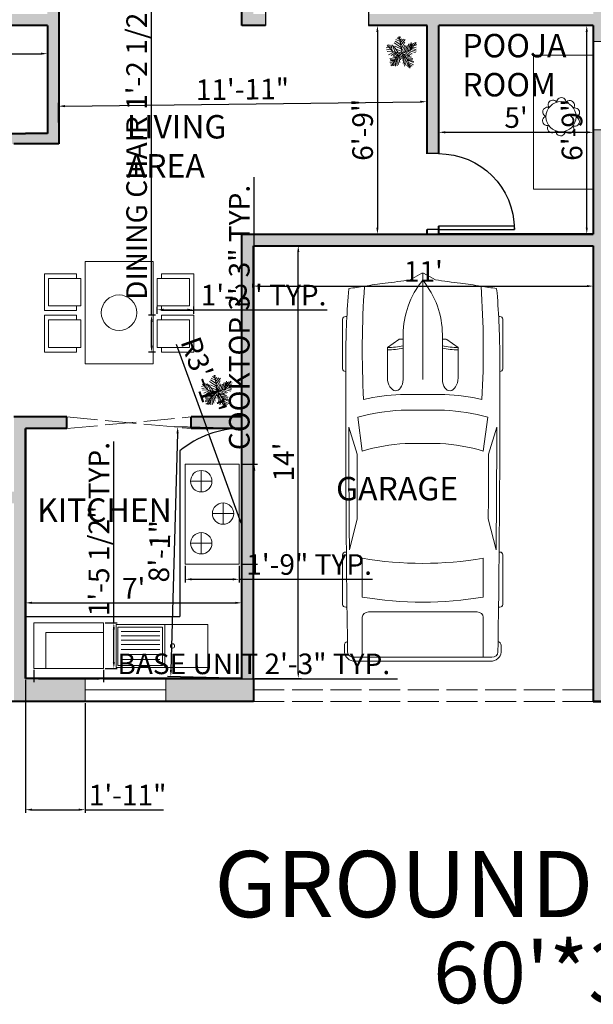
# Model space of a CAD drawing. Units: inches. Extents: x 529 to 1442, y 1029 to 1677.
# Tile 2 of 7: x 769 to 991, y 1029 to 1412. Entities that reach past the tile are written whole.
import ezdxf

# ---------------------------------------------------------------- set-up
doc = ezdxf.new("R2010")
doc.units = ezdxf.units.IN
doc.linetypes.add('ACAD_ISO02W100', pattern=[15, 12, -3])
for name, color, linetype, lineweight in [('A-ANNO-DIMS', 2, 'Continuous', 18), ('A-ANNO-TEXT', 7, 'Continuous', 30), ('A-AREA-IDEN', 7, 'Continuous', 25), ('A-DOOR', 4, 'Continuous', 25), ('A-EQPM-VEHL', 8, 'Continuous', 13), ('A-FLOR-CASE', 32, 'Continuous', 25), ('A-FLOR-FIXT', 9, 'Continuous', 18), ('A-FLOR-OVHD', 8, 'ACAD_ISO02W100', 18), ('A-FURN', 8, 'Continuous', 18), ('A-WALL-PATT', 252, 'Continuous', 13), ('kit', 10, 'Continuous', 18), ('pooja', 40, 'Continuous', 18), ('tree', 70, 'Continuous', 13), ('wall', 7, 'Continuous', 40), ('window', 52, 'Continuous', 18)]:
    doc.layers.add(name, color=color, linetype=linetype, lineweight=lineweight)
doc.styles.get("Standard").update_dxf_attribs({"font": 'arial.ttf'})
doc.dimstyles.new('ISO-25', dxfattribs={"dimtxt": 8, "dimasz": 2.5, "dimexe": 1.25, "dimexo": 0.625, "dimtad": 1, "dimdec": 0, "dimlunit": 4, "dimtxsty": 'Standard', "dimcen": 2.5, "dimadec": 0, "dimazin": 0, "dimtfac": 1, "dimtdec": 0, "dimtmove": 0, "dimatfit": 3, "dimfxl": 1, "dimarcsym": 0})

# ---------------------------------------------------------------- blocks, each defined once
blk = doc.blocks.new('*U2')
for p, q in [((0, 0), (0, -6)), ((40, 0), (40, -6))]:
    blk.add_line(p, q)
blk.add_lwpolyline([(0, 0), (0, 40), (1.75, 40), (1.75, 0)], close=True)
blk.add_arc((0, 0), 40, 0, 90)
blk = doc.blocks.new('*U6')
for p, q in [((46.55, 38.89), (22.35, 38.89)), ((136.7, 38.89), (160.9, 38.89)), ((21.1, 37.41), (21.1, 36.83)), ((47.8, 37.39), (47.8, 37.41)), ((87.99, 31.87), (74.76, 35.92)), ((134.31, 35.6), (119.29, 31.78)), ((135.45, 37.07), (135.45, 37.41)), ((162.15, 37.41), (162.15, 36.77)), ((186.47, -33.5), (186.47, 33.5)), ((70.03, 31.54), (86.41, 29.35)), ((138.42, 29.35), (157.25, 29.35)), ((186.47, 29.35), (167.01, 29.35)), ((188.4, -32.76), (188.4, 32.76)), ((164.52, 26.39), (164.52, -26.39)), ((32.27, 11.63), (36.13, 17.17)), ((36.13, 17.17), (50.94, 17.17)), ((32.12, 9.51), (32.12, 11.15)), ((58.92, -10.77), (58.92, 10.77)), ((66.55, -10.53), (66.55, 10.53)), ((186.47, -10.53), (186.47, 10.53)), ((3.27, 6.13), (0.1, 0.41)), ((29.77, 9.51), (51.68, 9.51)), ((82.74, 8.5), (82.74, -8.5)), ((0, 0), (51.68, 0)), ((0.1, -0.41), (3.27, -6.13)), ((29.77, -9.51), (51.68, -9.51)), ((32.12, -9.51), (32.12, -11.15)), ((32.27, -11.63), (36.13, -17.17)), ((36.13, -17.17), (50.94, -17.17)), ((86.41, -29.35), (70.03, -31.54)), ((87.99, -31.87), (74.76, -35.92)), ((134.31, -35.6), (119.29, -31.78)), ((157.25, -29.35), (138.42, -29.35)), ((167.01, -29.35), (186.47, -29.35)), ((21.1, -37.41), (21.1, -36.83)), ((47.8, -37.39), (47.8, -37.41)), ((135.45, -37.07), (135.45, -37.41)), ((162.15, -37.41), (162.15, -36.77)), ((46.55, -38.89), (22.35, -38.89)), ((136.7, -38.89), (160.9, -38.89))]:
    blk.add_line(p, q)
for centre, major_axis, ratio, start_param, end_param in [((22.35, 37.41), (0, -1.48), 0.842304, 3.141593, 4.712389), ((46.55, 37.41), (0, 1.48), 0.842304, -1.570796, 0), ((136.7, 37.41), (0, -1.48), 0.842304, 3.141593, 4.712389), ((160.9, 37.41), (0, 1.48), 0.842304, -1.570796, 0), ((266.03, -27.52), (0, 313.31), 0.842304, 1.367076, 1.39176), ((41.19, -490.86), (0, 528.23), 0.842304, 0.00281, 0.075598), ((64.48, -10555.62), (0, 10593.03), 0.842304, -0.013397, 0.002797), ((64.48, -10555.62), (0, -10591.55), 0.842304, 3.133765, 3.140441), ((180.63, 35.84), (0, 2.22), 0.842304, -0.013017, 1.249894), ((64.48, -10556.36), (0, 10595.31), 0.842304, -0.013397, -0.013017), ((183.98, 33.5), (0, -2.96), 0.842304, 1.570796, 3.128196), ((183.98, 32.76), (0, -5.25), 0.842304, 1.570796, 3.128196), ((37.47, -593.96), (0, -623.33), 0.842304, 3.096046, 3.200911), ((134.4, 5.39), (0, -89.78), 0.842304, 4.449482, 4.652344), ((135.29, 5.39), (0, 81.77), 0.842304, 1.245306, 1.50788), ((149.6, 2.8), (0, -79.58), 0.842304, 4.372215, 4.640744), ((95.79, -3666.35), (0, -3698.24), 0.842304, 3.134049, 3.144098), ((17.08, 0), (0, 147.02), 0.842304, 4.511394, 4.913384), ((35.91, 0), (0, 147.02), 0.842304, 4.511394, 4.913384), ((167.01, 26.39), (0, 2.96), 0.842304, 0, 1.570796), ((259.18, -27.52), (0, -305.3), 0.842304, 4.528606, 4.561838), ((-204.49, 52.4), (0, -250.96), 0.842304, 1.385369, 1.434372), ((13.04, 17.01), (0, 27.42), 0.842304, 4.435146, 4.718221), ((14.2, 17.01), (0, 27.42), 0.842304, 4.435146, 4.718221), ((50.79, 13.34), (6.34, -0.36), 0.603834, -1.395552, 1.581315), ((32.75, 11.15), (0, 0.74), 0.842304, 0.879714, 1.570796), ((29.77, -46.66), (0, 56.17), 0.842304, 0, 0.590319), ((0.62, 0), (0, -0.74), 0.842304, 4.131459, 5.293319), ((29.77, 46.66), (0, 56.17), 0.842304, 2.551274, 3.141593), ((-204.49, -52.4), (0, 250.96), 0.842304, -1.434372, -1.385369), ((13.04, -17.01), (0, -27.42), 0.842304, 1.564964, 1.848039), ((14.2, -17.01), (0, -27.42), 0.842304, 1.564964, 1.848039), ((149.6, -2.8), (0, -79.58), 0.842304, -1.499151, -1.230623), ((32.75, -11.15), (0, -0.74), 0.842304, 4.712389, 5.403472), ((134.4, -5.39), (0, -89.78), 0.842304, -1.510751, -1.307889), ((135.29, -5.39), (0, -81.77), 0.842304, -1.50788, -1.245306), ((259.18, 27.52), (0, 305.3), 0.842304, 1.721348, 1.754579), ((266.03, 27.52), (0, 313.31), 0.842304, 1.749832, 1.774517), ((37.47, 593.96), (0, -623.33), 0.842304, -0.059319, 0.045547), ((167.01, -26.39), (0, -2.96), 0.842304, 4.712389, 6.283185), ((95.79, 3666.35), (0, -3698.24), 0.842304, -0.002505, 0.007544), ((183.98, -32.76), (0, -5.25), 0.842304, 0.013397, 1.570796), ((41.19, 490.86), (0, -528.23), 0.842304, -0.075598, -0.00281), ((22.35, -37.41), (0, 1.48), 0.842304, 1.570796, 3.141593), ((64.48, 10555.62), (0, 10593.03), 0.842304, 3.138796, 3.15499), ((46.55, -37.41), (0, -1.48), 0.842304, 0, 1.570796), ((64.48, 10555.62), (0, -10591.55), 0.842304, 0.001152, 0.007828), ((136.7, -37.41), (0, -1.48), 0.842304, -1.570796, 0), ((160.9, -37.41), (0, 1.48), 0.842304, 3.141593, 4.712389), ((180.63, -35.84), (0, -2.22), 0.842304, -1.249894, 0.013017), ((64.48, 10556.36), (0, 10595.31), 0.842304, 3.15461, 3.15499), ((183.98, -33.5), (0, 2.96), 0.842304, 3.15499, 4.712389)]:
    blk.add_ellipse(centre, major_axis=major_axis, ratio=ratio, start_param=start_param, end_param=end_param)
at = {"extrusion": (0, 0, -1)}
blk.add_ellipse((50.79, -13.34), major_axis=(6.34, 0.36), ratio=0.603834, start_param=-1.395552, end_param=1.581315, dxfattribs=at)
blk = doc.blocks.new('*U9')
blk.add_circle((0, -0.78), 5.87)
blk.add_arc((0.14, 4.85), 1.8, 357.1489, 180)
blk = doc.blocks.new('*U10')
at = {"layer": 'pooja', "transparency": 16777216}
for p, rotation in [((1336.39, 1386.05), 36), ((1336.39, 1384.79), 144), ((1336.11, 1385.66), 72), ((1336.11, 1385.18), 108), ((1337.31, 1386.05), 324.0000000000001), ((1337.31, 1384.79), 216), ((1337.6, 1385.66), 288), ((1337.6, 1385.18), 252), ((1336.85, 1384.64), 180)]:
    blk.add_blockref('*U9', p, dxfattribs=dict(at, rotation=rotation))
blk.add_blockref('*U9', (1336.85, 1386.2), dxfattribs=at)
blk = doc.blocks.new('*U12')
for p, q in [((-3.665, 19.273), (-27.574, 35.527)), ((-5.114, 28.097), (-24.676, 40.636)), ((-7.288, 39.707), (-21.778, 46.673)), ((-8.737, 47.138), (-17.069, 52.711)), ((-10.186, 53.64), (-13.084, 55.962)), ((0, 0), (-10.5, 57)), ((-9.099, 51.782), (-6.563, 55.962)), ((-7.65, 43.423), (-2.578, 49.46)), ((-5.839, 35.992), (4.667, 48.067)), ((-5.114, 27.632), (10.463, 46.673)), ((-2.941, 16.486), (8.652, 37.85)), ((27, 9), (48, 36)), ((27.127, 9.056), (31.112, 35.992)), ((44.153, 36.456), (45.239, 32.741)), ((-47.498, 19.737), (-55.83, 18.344)), ((-40.615, 13.7), (-55.105, 10.913)), ((-31.5, 4.5), (-52.5, 25.5)), ((-33.37, 6.269), (-52.207, 5.34)), ((-48.585, 21.131), (-49.309, 29.026)), ((-28.299, 3.483), (-47.86, -5.805)), ((-43.513, 28.561), (-42.427, 15.558)), ((-38.442, 26.239), (-34.819, 7.663)), ((-21.416, 3.018), (-38.079, -8.128)), ((-35.544, 28.097), (-24.314, 3.947)), ((0, 0), (-31.5, 4.5)), ((-14.533, 2.09), (-30.834, 25.31)), ((-15.982, 2.09), (-30.11, -9.521)), ((-24.314, 23.917), (-2.941, 13.7)), ((0, 0), (-22.5, -19.5)), ((-6.563, 1.161), (-21.416, -8.128)), ((-20.691, 13.7), (-1.129, 4.876)), ((-1.129, 6.734), (9.014, 26.704)), ((0, 0), (27, 9)), ((0, 0), (18, -22.5)), ((3.942, 1.625), (11.187, 24.381)), ((6.478, 1.625), (26.04, -8.592)), ((10.101, 3.483), (17.708, 26.239)), ((11.187, 3.483), (30.749, -5.805)), ((16.259, 5.805), (23.142, 31.348)), ((18.07, 5.805), (35.096, -3.483)), ((22.055, 7.198), (27.489, 32.277)), ((24.229, 7.663), (46.688, 1.625)), ((29.662, 12.307), (48.137, 6.269)), ((31.836, 30.883), (32.561, 16.486)), ((33.285, 16.486), (48.862, 10.913)), ((35.096, 32.741), (37.27, 22.524)), ((36.183, 19.737), (48.137, 17.88)), ((38.719, 34.134), (41.979, 28.561)), ((40.53, 25.775), (48.862, 24.846)), ((43.791, 29.954), (51.036, 30.883)), ((-17.431, -15.094), (-42.789, -18.809)), ((-28.299, -29.026), (-42.789, -31.348)), ((-24.314, -21.596), (-42.427, -22.06)), ((-30.834, -34.135), (-42.427, -35.528)), ((-26.849, -26.24), (-40.253, -25.775)), ((-22.5, -19.5), (-37.5, -45)), ((-15.257, -12.772), (-30.11, -12.772)), ((-29.023, -30.884), (-27.936, -43.887)), ((-25.038, -23.918), (-22.865, -45.281)), ((-20.691, -18.345), (-17.793, -44.352)), ((-6.563, -5.805), (-19.967, -9.985)), ((-17.069, -15.094), (-12.721, -40.172)), ((-13.446, -11.378), (-8.737, -32.741)), ((-9.461, -8.592), (-6.201, -23.453)), ((-4.752, -3.483), (-3.665, -14.629)), ((2.493, -3.019), (-1.491, -20.202)), ((1.769, -2.555), (24.229, -9.521)), ((5.029, -6.27), (2.131, -25.775)), ((9.014, -11.378), (3.58, -35.992)), ((14.085, -16.951), (6.478, -40.172)), ((7.565, -9.056), (32.198, -14.629)), ((18.07, -22.524), (8.289, -45.745)), ((12.274, -15.094), (36.907, -18.809)), ((20.244, -30.419), (15.897, -44.816)), ((16.259, -19.738), (36.183, -22.989)), ((18, -22.5), (27, -52.5)), ((18.433, -22.524), (40.53, -29.026)), ((19.157, -25.311), (38.719, -33.206)), ((21.331, -32.741), (39.081, -40.636)), ((-34.457, -39.708), (-40.978, -42.494)), ((-32.646, -36.921), (-31.921, -44.352)), ((22.78, -37.85), (19.519, -48.532)), ((22.78, -38.314), (34.372, -44.816)), ((24.591, -45.745), (23.142, -50.854)), ((24.591, -43.423), (30.749, -47.603)), ((26.764, -49.925), (28.213, -50.854))]:
    blk.add_line(p, q)
blk = doc.blocks.new('*D35')
at = {"layer": 'A-ANNO-DIMS', "color": 0, "lineweight": -2, "transparency": 16777216}
for p, q in [((860.01, 1323.81), (878.07, 1323.81)), ((876.82, 1158.31), (876.82, 1321.31)), ((860.01, 1155.81), (878.07, 1155.81))]:
    blk.add_line(p, q, dxfattribs=at)
at = {"layer": 'A-ANNO-DIMS', "color": 0, "lineweight": 100, "transparency": 16777216}
for points in [[(876.41, 1321.31), (877.24, 1321.31), (876.82, 1323.81)], [(876.41, 1158.31), (877.24, 1158.31), (876.82, 1155.81)]]:
    blk.add_solid(points, dxfattribs=at)
at = {"layer": 'Defpoints', "color": 0, "lineweight": 100, "transparency": 16777216}
for p in [(859.38, 1323.81), (876.82, 1323.81), (859.38, 1155.81)]:
    blk.add_point(p, dxfattribs=at)
at = {"layer": 'A-ANNO-DIMS', "color": 0, "transparency": 16777216, "insert": (872.18, 1239.81), "char_height": 8, "attachment_point": 5, "rotation": 90}
blk.add_mtext("14'", dxfattribs=at)
blk = doc.blocks.new('*D36')
at = {"layer": 'A-ANNO-DIMS', "color": 0, "lineweight": -2, "transparency": 16777216}
for p, q in [((859.38, 1323.19), (859.38, 1306.86)), ((991.38, 1323.19), (991.38, 1306.86)), ((861.88, 1308.11), (988.88, 1308.11))]:
    blk.add_line(p, q, dxfattribs=at)
at = {"layer": 'A-ANNO-DIMS', "color": 0, "lineweight": 100, "transparency": 16777216}
for points in [[(861.88, 1308.53), (861.88, 1307.7), (859.38, 1308.11)], [(988.88, 1308.53), (988.88, 1307.7), (991.38, 1308.11)]]:
    blk.add_solid(points, dxfattribs=at)
at = {"layer": 'Defpoints', "color": 0, "lineweight": 100, "transparency": 16777216}
for p in [(859.38, 1323.81), (991.38, 1323.81), (991.38, 1308.11)]:
    blk.add_point(p, dxfattribs=at)
at = {"layer": 'A-ANNO-DIMS', "color": 0, "transparency": 16777216, "insert": (925.38, 1312.76), "char_height": 8, "attachment_point": 5}
blk.add_mtext("11'", dxfattribs=at)
blk = doc.blocks.new('*D37')
at = {"layer": 'A-ANNO-DIMS', "color": 0, "lineweight": -2, "transparency": 16777216}
for p, q in [((770.88, 1156.44), (770.88, 1186.38)), ((854.88, 1156.44), (854.88, 1186.38)), ((773.38, 1185.13), (852.38, 1185.13))]:
    blk.add_line(p, q, dxfattribs=at)
at = {"layer": 'A-ANNO-DIMS', "color": 0, "lineweight": 100, "transparency": 16777216}
for points in [[(773.38, 1185.55), (773.38, 1184.72), (770.88, 1185.13)], [(852.38, 1185.55), (852.38, 1184.72), (854.88, 1185.13)]]:
    blk.add_solid(points, dxfattribs=at)
at = {"layer": 'Defpoints', "color": 0, "lineweight": 100, "transparency": 16777216}
for p in [(854.88, 1185.13), (770.88, 1155.81), (854.88, 1155.81)]:
    blk.add_point(p, dxfattribs=at)
at = {"layer": 'A-ANNO-DIMS', "color": 0, "transparency": 16777216, "insert": (812.88, 1189.76), "char_height": 8, "attachment_point": 5}
blk.add_mtext("7'", dxfattribs=at)
blk = doc.blocks.new('*D38')
at = {"layer": 'A-ANNO-DIMS', "color": 0, "lineweight": -2, "transparency": 16777216}
for p, q in [((829.93, 1250.99), (827.39, 1158.98)), ((853.74, 1252.83), (828.75, 1253.52)), ((851.06, 1155.83), (826.07, 1156.52))]:
    blk.add_line(p, q, dxfattribs=at)
at = {"layer": 'A-ANNO-DIMS', "color": 0, "lineweight": 100, "transparency": 16777216}
for points in [[(829.52, 1251), (830.35, 1250.97), (830, 1253.49)], [(826.97, 1159), (827.81, 1158.97), (827.32, 1156.49)]]:
    blk.add_solid(points, dxfattribs=at)
at = {"layer": 'Defpoints', "color": 0, "lineweight": 100, "transparency": 16777216}
for p in [(854.36, 1252.81), (827.32, 1156.49), (851.69, 1155.81)]:
    blk.add_point(p, dxfattribs=at)
at = {"layer": 'A-ANNO-DIMS', "color": 0, "transparency": 16777216, "insert": (823.95, 1205.12), "char_height": 8, "attachment_point": 5, "rotation": 88.418}
blk.add_mtext('8\'-1"', dxfattribs=at)
blk = doc.blocks.new('*D43')
at = {"layer": 'A-ANNO-DIMS', "color": 0, "lineweight": -2, "transparency": 16777216}
for p, q in [((926.88, 1365.7), (926.69, 1380.98)), ((783.88, 1363.94), (783.69, 1379.22)), ((786.2, 1378), (924.2, 1379.7))]:
    blk.add_line(p, q, dxfattribs=at)
at = {"layer": 'A-ANNO-DIMS', "color": 0, "lineweight": 100, "transparency": 16777216}
for points in [[(786.2, 1378.42), (786.21, 1377.58), (783.7, 1377.97)], [(924.2, 1380.12), (924.21, 1379.29), (926.7, 1379.73)]]:
    blk.add_solid(points, dxfattribs=at)
at = {"layer": 'Defpoints', "color": 0, "lineweight": 100, "transparency": 16777216}
for p in [(926.7, 1379.73), (926.88, 1365.08), (783.88, 1363.31)]:
    blk.add_point(p, dxfattribs=at)
at = {"layer": 'A-ANNO-DIMS', "color": 0, "transparency": 16777216, "insert": (855.15, 1383.49), "char_height": 8, "attachment_point": 5, "rotation": 0.7072}
blk.add_mtext('11\'-11"', dxfattribs=at)
blk = doc.blocks.new('*D44')
at = {"layer": 'A-ANNO-DIMS', "color": 0, "lineweight": -2, "transparency": 16777216}
for p, q in [((926.26, 1409.31), (906.3, 1409.31)), ((907.55, 1406.81), (907.55, 1330.81)), ((926.26, 1328.31), (906.3, 1328.31))]:
    blk.add_line(p, q, dxfattribs=at)
at = {"layer": 'A-ANNO-DIMS', "color": 0, "lineweight": 100, "transparency": 16777216}
for points in [[(907.13, 1406.81), (907.96, 1406.81), (907.55, 1409.31)], [(907.13, 1330.81), (907.96, 1330.81), (907.55, 1328.31)]]:
    blk.add_solid(points, dxfattribs=at)
at = {"layer": 'Defpoints', "color": 0, "lineweight": 100, "transparency": 16777216}
for p in [(926.88, 1409.31), (907.55, 1328.31), (926.88, 1328.31)]:
    blk.add_point(p, dxfattribs=at)
at = {"layer": 'A-ANNO-DIMS', "color": 0, "transparency": 16777216, "insert": (902.84, 1368.81), "char_height": 8, "attachment_point": 5, "rotation": 90}
blk.add_mtext('6\'-9"', dxfattribs=at)
blk = doc.blocks.new('*D45')
at = {"layer": 'A-ANNO-DIMS', "color": 0, "lineweight": -2, "transparency": 16777216}
for p, q in [((647.38, 1408.69), (647.38, 1397.12)), ((779.38, 1408.69), (779.38, 1397.12)), ((649.88, 1398.37), (776.88, 1398.37))]:
    blk.add_line(p, q, dxfattribs=at)
at = {"layer": 'A-ANNO-DIMS', "color": 0, "lineweight": 100, "transparency": 16777216}
for points in [[(649.88, 1398.78), (649.88, 1397.95), (647.38, 1398.37)], [(776.88, 1398.78), (776.88, 1397.95), (779.38, 1398.37)]]:
    blk.add_solid(points, dxfattribs=at)
at = {"layer": 'Defpoints', "color": 0, "lineweight": 100, "transparency": 16777216}
for p in [(647.38, 1409.31), (779.38, 1409.31), (779.38, 1398.37)]:
    blk.add_point(p, dxfattribs=at)
at = {"layer": 'A-ANNO-DIMS', "color": 0, "transparency": 16777216, "insert": (713.38, 1403.01), "char_height": 8, "attachment_point": 5}
blk.add_mtext("11'", dxfattribs=at)
blk = doc.blocks.new('*D47')
at = {"layer": 'A-ANNO-DIMS', "color": 0, "lineweight": -2, "transparency": 16777216}
for p, q in [((931.38, 1408.69), (931.38, 1366.59)), ((991.38, 1408.69), (991.38, 1366.59)), ((933.88, 1367.84), (988.88, 1367.84))]:
    blk.add_line(p, q, dxfattribs=at)
at = {"layer": 'A-ANNO-DIMS', "color": 0, "lineweight": 100, "transparency": 16777216}
for points in [[(933.88, 1368.25), (933.88, 1367.42), (931.38, 1367.84)], [(988.88, 1368.25), (988.88, 1367.42), (991.38, 1367.84)]]:
    blk.add_solid(points, dxfattribs=at)
at = {"layer": 'Defpoints', "color": 0, "lineweight": 100, "transparency": 16777216}
for p in [(931.38, 1409.31), (991.38, 1409.31), (991.38, 1367.84)]:
    blk.add_point(p, dxfattribs=at)
at = {"layer": 'A-ANNO-DIMS', "color": 0, "transparency": 16777216, "insert": (961.38, 1372.53), "char_height": 8, "attachment_point": 5}
blk.add_mtext("5'", dxfattribs=at)
blk = doc.blocks.new('*D48')
at = {"layer": 'A-ANNO-DIMS', "color": 0, "lineweight": -2, "transparency": 16777216}
for p, q in [((990.76, 1409.31), (987.59, 1409.31)), ((988.84, 1330.81), (988.84, 1406.81)), ((990.76, 1328.31), (987.59, 1328.31))]:
    blk.add_line(p, q, dxfattribs=at)
at = {"layer": 'A-ANNO-DIMS', "color": 0, "lineweight": 100, "transparency": 16777216}
for points in [[(988.43, 1406.81), (989.26, 1406.81), (988.84, 1409.31)], [(988.43, 1330.81), (989.26, 1330.81), (988.84, 1328.31)]]:
    blk.add_solid(points, dxfattribs=at)
at = {"layer": 'Defpoints', "color": 0, "lineweight": 100, "transparency": 16777216}
for p in [(988.84, 1409.31), (991.38, 1409.31), (991.38, 1328.31)]:
    blk.add_point(p, dxfattribs=at)
at = {"layer": 'A-ANNO-DIMS', "color": 0, "transparency": 16777216, "insert": (984.14, 1368.81), "char_height": 8, "attachment_point": 5, "rotation": 90}
blk.add_mtext('6\'-9"', dxfattribs=at)
blk = doc.blocks.new('WIN-SMALL-PLAN')
blk.add_line((0, 4.5), (31.29, 4.5))
blk.add_lwpolyline([(0, 9), (31.29, 9), (31.29, 0), (0, 0)], close=True)
blk = doc.blocks.new('DINING-CHAIR')
for p, q in [((1.76, 12.47), (1.76, 14.29)), ((1.76, 14.29), (14.22, 14.29)), ((14.22, 14.29), (14.22, 0)), ((1.76, 0), (1.76, 1.83)), ((14.22, 0), (1.76, 0))]:
    blk.add_line(p, q)
blk.add_lwpolyline([(0, 12.47), (12.59, 12.47), (12.59, 1.83), (0, 1.83)], close=True)
blk = doc.blocks.new('DINING-TABLE')
blk.add_lwpolyline([(26.42, 39.82), (0, 39.82), (0, 0), (26.42, 0)], close=True)
blk.add_circle((13.21, 19.91), 6.89)
blk = doc.blocks.new('KITCHEN-COUNTER-UNIT')
for p, q in [((4.66, 0), (4.66, 13.96)), ((4.66, 13.96), (26.96, 13.96))]:
    blk.add_line(p, q)
blk.add_lwpolyline([(0, 17.63), (26.96, 17.63), (26.96, 0), (0, 0)], close=True)
blk = doc.blocks.new('SINK-WITH-DRAINBOARD')
for p, q in [((18.91, 0), (18.91, 16.76)), ((1.96, 14.02), (16.96, 14.02)), ((1.96, 12.32), (16.96, 12.32)), ((1.96, 10.57), (16.96, 10.57)), ((1.96, 8.97), (16.96, 8.97)), ((1.96, 7.02), (16.96, 7.02)), ((1.96, 5.06), (16.96, 5.06)), ((1.96, 3.1), (16.96, 3.1))]:
    blk.add_line(p, q)
for points in [[(0, 0), (35.68, 0), (35.68, 16.76), (0, 16.76)], [(0.77, 15.62), (18.04, 15.62), (18.04, 0.78), (0.77, 0.78)]]:
    blk.add_lwpolyline(points, close=True)
blk.add_circle((21.95, 8.38), 0.822)
blk = doc.blocks.new('COOKTOP-THREE-BURNER')
for p, q in [((6.23, 28.11), (6.23, 36.44)), ((6.23, 36.44), (6.23, 32.27)), ((10.39, 32.27), (2.07, 32.27)), ((6.23, 32.27), (10.39, 32.27)), ((14.71, 15.52), (14.71, 23.85)), ((14.71, 23.85), (14.71, 19.68)), ((18.87, 19.68), (10.54, 19.68)), ((14.71, 19.68), (18.87, 19.68)), ((6.23, 3.99), (6.23, 12.32)), ((6.23, 12.32), (6.23, 8.16)), ((10.39, 8.16), (2.07, 8.16)), ((6.23, 8.16), (10.39, 8.16))]:
    blk.add_line(p, q)
blk.add_lwpolyline([(0, 38.87), (20.99, 38.87), (20.99, 0), (0, 0)], close=True)
for centre in [(6.23, 32.27), (14.71, 19.68), (6.23, 8.16)]:
    blk.add_circle(centre, 4.16)
blk = doc.blocks.new('*D81')
at = {"layer": 'A-ANNO-DIMS', "color": 0, "lineweight": -2, "transparency": 16777216}
for p, q in [((819.84, 1296.79), (819.84, 1447.64)), ((821.36, 1296.79), (818.59, 1296.79)), ((819.84, 1285), (819.84, 1294.29)), ((821.36, 1282.5), (818.59, 1282.5))]:
    blk.add_line(p, q, dxfattribs=at)
at = {"layer": 'A-ANNO-DIMS', "color": 0, "lineweight": 100, "transparency": 16777216}
for points in [[(819.43, 1294.29), (820.26, 1294.29), (819.84, 1296.79)], [(819.43, 1285), (820.26, 1285), (819.84, 1282.5)]]:
    blk.add_solid(points, dxfattribs=at)
at = {"layer": 'Defpoints', "color": 0, "lineweight": 100, "transparency": 16777216}
for p in [(819.84, 1296.79), (821.99, 1296.79), (821.99, 1282.5)]:
    blk.add_point(p, dxfattribs=at)
at = {"layer": 'A-ANNO-DIMS', "color": 0, "transparency": 16777216, "insert": (815.08, 1373.47), "char_height": 8, "attachment_point": 5, "rotation": 90}
blk.add_mtext('DINING CHAIR 1\'-2 1/2" TYP.', dxfattribs=at)
blk = doc.blocks.new('*D82')
at = {"layer": 'A-ANNO-DIMS', "color": 0, "lineweight": -2, "transparency": 16777216}
for p, q in [((821.99, 1297.41), (821.99, 1300.18)), ((836.21, 1297.41), (836.21, 1300.18)), ((824.49, 1298.93), (833.71, 1298.93)), ((836.21, 1298.93), (887.97, 1298.93))]:
    blk.add_line(p, q, dxfattribs=at)
at = {"layer": 'A-ANNO-DIMS', "color": 0, "lineweight": 100, "transparency": 16777216}
for points in [[(824.49, 1299.35), (824.49, 1298.52), (821.99, 1298.93)], [(833.71, 1299.35), (833.71, 1298.52), (836.21, 1298.93)]]:
    blk.add_solid(points, dxfattribs=at)
at = {"layer": 'Defpoints', "color": 0, "lineweight": 100, "transparency": 16777216}
for p in [(821.99, 1296.79), (836.21, 1298.93), (836.21, 1296.79)]:
    blk.add_point(p, dxfattribs=at)
at = {"layer": 'A-ANNO-DIMS', "color": 0, "transparency": 16777216, "insert": (863.34, 1303.58), "char_height": 8, "attachment_point": 5}
blk.add_mtext('1\'-2" TYP.', dxfattribs=at)
blk = doc.blocks.new('*D93')
at = {"layer": 'A-ANNO-DIMS', "color": 0, "lineweight": -2, "transparency": 16777216}
for p, q in [((774.19, 1159.06), (774.19, 1154.39)), ((801.15, 1159.06), (801.15, 1154.39)), ((776.69, 1155.64), (798.65, 1155.64)), ((801.15, 1155.64), (915.41, 1155.64))]:
    blk.add_line(p, q, dxfattribs=at)
at = {"layer": 'A-ANNO-DIMS', "color": 0, "lineweight": 100, "transparency": 16777216}
for points in [[(776.69, 1156.05), (776.69, 1155.22), (774.19, 1155.64)], [(798.65, 1156.05), (798.65, 1155.22), (801.15, 1155.64)]]:
    blk.add_solid(points, dxfattribs=at)
at = {"layer": 'Defpoints', "color": 0, "lineweight": 100, "transparency": 16777216}
for p in [(774.19, 1159.68), (801.15, 1159.68), (801.15, 1155.64)]:
    blk.add_point(p, dxfattribs=at)
at = {"layer": 'A-ANNO-DIMS', "color": 0, "transparency": 16777216, "insert": (859.53, 1160.4), "char_height": 8, "attachment_point": 5}
blk.add_mtext('BASE UNIT 2\'-3" TYP.', dxfattribs=at)
blk = doc.blocks.new('*D94')
at = {"layer": 'A-ANNO-DIMS', "color": 0, "lineweight": -2, "transparency": 16777216}
for p, q in [((805.2, 1177.31), (805.2, 1247.72)), ((801.78, 1177.31), (806.45, 1177.31)), ((805.2, 1162.18), (805.2, 1174.81)), ((801.78, 1159.68), (806.45, 1159.68))]:
    blk.add_line(p, q, dxfattribs=at)
at = {"layer": 'A-ANNO-DIMS', "color": 0, "lineweight": 100, "transparency": 16777216}
for points in [[(804.78, 1174.81), (805.61, 1174.81), (805.2, 1177.31)], [(804.78, 1162.18), (805.61, 1162.18), (805.2, 1159.68)]]:
    blk.add_solid(points, dxfattribs=at)
at = {"layer": 'Defpoints', "color": 0, "lineweight": 100, "transparency": 16777216}
for p in [(801.15, 1177.31), (805.2, 1177.31), (801.15, 1159.68)]:
    blk.add_point(p, dxfattribs=at)
at = {"layer": 'A-ANNO-DIMS', "color": 0, "transparency": 16777216, "insert": (800.44, 1213.76), "char_height": 8, "attachment_point": 5, "rotation": 90}
blk.add_mtext('1\'-5 1/2" TYP.', dxfattribs=at)
blk = doc.blocks.new('*D97')
at = {"layer": 'A-ANNO-DIMS', "color": 0, "lineweight": -2, "transparency": 16777216}
for p, q in [((859.72, 1238.97), (859.72, 1350.38)), ((854.52, 1238.97), (860.97, 1238.97)), ((859.72, 1202.6), (859.72, 1236.47)), ((854.52, 1200.1), (860.97, 1200.1))]:
    blk.add_line(p, q, dxfattribs=at)
at = {"layer": 'A-ANNO-DIMS', "color": 0, "lineweight": 100, "transparency": 16777216}
for points in [[(859.3, 1236.47), (860.14, 1236.47), (859.72, 1238.97)], [(859.3, 1202.6), (860.14, 1202.6), (859.72, 1200.1)]]:
    blk.add_solid(points, dxfattribs=at)
at = {"layer": 'Defpoints', "color": 0, "lineweight": 100, "transparency": 16777216}
for p in [(853.89, 1238.97), (859.72, 1238.97), (853.89, 1200.1)]:
    blk.add_point(p, dxfattribs=at)
at = {"layer": 'A-ANNO-DIMS', "color": 0, "transparency": 16777216, "insert": (854.95, 1295.93), "char_height": 8, "attachment_point": 5, "rotation": 90}
blk.add_mtext('COOKTOP 3\'-3" TYP.', dxfattribs=at)
blk = doc.blocks.new('*D98')
at = {"layer": 'A-ANNO-DIMS', "color": 0, "lineweight": -2, "transparency": 16777216}
for p, q in [((832.9, 1199.47), (832.9, 1193.02)), ((853.89, 1199.47), (853.89, 1193.02)), ((835.4, 1194.27), (851.39, 1194.27)), ((853.89, 1194.27), (905.65, 1194.27))]:
    blk.add_line(p, q, dxfattribs=at)
at = {"layer": 'A-ANNO-DIMS', "color": 0, "lineweight": 100, "transparency": 16777216}
for points in [[(835.4, 1194.68), (835.4, 1193.85), (832.9, 1194.27)], [(851.39, 1194.68), (851.39, 1193.85), (853.89, 1194.27)]]:
    blk.add_solid(points, dxfattribs=at)
at = {"layer": 'Defpoints', "color": 0, "lineweight": 100, "transparency": 16777216}
for p in [(832.9, 1200.1), (853.89, 1200.1), (853.89, 1194.27)]:
    blk.add_point(p, dxfattribs=at)
at = {"layer": 'A-ANNO-DIMS', "color": 0, "transparency": 16777216, "insert": (881.02, 1198.98), "char_height": 8, "attachment_point": 5}
blk.add_mtext('1\'-9" TYP.', dxfattribs=at)
blk = doc.blocks.new('*D111')
at = {"layer": 'A-ANNO-DIMS', "color": 0, "lineweight": -2, "transparency": 16777216}
for p, q in [((770.88, 1155.19), (770.88, 1103.56)), ((794.05, 1146.19), (794.05, 1103.56)), ((773.38, 1104.81), (791.55, 1104.81)), ((794.05, 1104.81), (824.53, 1104.81))]:
    blk.add_line(p, q, dxfattribs=at)
at = {"layer": 'A-ANNO-DIMS', "color": 0, "lineweight": 100, "transparency": 16777216}
for points in [[(773.38, 1105.23), (773.38, 1104.4), (770.88, 1104.81)], [(791.55, 1105.23), (791.55, 1104.4), (794.05, 1104.81)]]:
    blk.add_solid(points, dxfattribs=at)
at = {"layer": 'Defpoints', "color": 0, "lineweight": 100, "transparency": 16777216}
for p in [(770.88, 1155.81), (794.05, 1146.81), (794.05, 1104.81)]:
    blk.add_point(p, dxfattribs=at)
at = {"layer": 'A-ANNO-DIMS', "color": 0, "transparency": 16777216, "insert": (810.54, 1109.45), "char_height": 8, "attachment_point": 5}
blk.add_mtext('1\'-11"', dxfattribs=at)
blk = doc.blocks.new('*D118')
at = {"layer": 'A-ANNO-DIMS', "color": 0, "lineweight": -2, "transparency": 16777216}
for p, q in [((829.46, 1285.55), (841.25, 1252.97)), ((854.62, 1216.04), (842.11, 1250.62))]:
    blk.add_line(p, q, dxfattribs=at)
at = {"layer": 'A-ANNO-DIMS', "color": 0, "lineweight": 100, "transparency": 16777216}
blk.add_solid([(841.65, 1253.11), (840.86, 1252.83), (842.11, 1250.62)], dxfattribs=at)
at = {"layer": 'Defpoints', "color": 0, "lineweight": 100, "transparency": 16777216}
for p in [(842.11, 1250.62), (854.62, 1216.04)]:
    blk.add_point(p, dxfattribs=at)
at = {"layer": 'A-ANNO-DIMS', "color": 0, "transparency": 16777216, "insert": (839.03, 1272.97), "char_height": 8, "attachment_point": 5, "rotation": 289.9001}
blk.add_mtext('R3\'-1"', dxfattribs=at)

msp = doc.modelspace()

# ---------------------------------------------------------------- hatches: boundary and pattern name
at = {"layer": 'A-WALL-PATT'}
h = msp.add_hatch(color=256, dxfattribs=at)
h.dxf.hatch_style = 1
h.paths.add_polyline_path([(678.78, 1566.81), (638.38, 1566.81), (638.38, 1489.81), (647.38, 1489.81), (647.38, 1557.81), (678.78, 1557.81)])
h.paths.add_polyline_path([(805.14, 1566.81), (747.64, 1566.81), (747.64, 1557.81), (779.38, 1557.81), (805.14, 1557.81)])
h.paths.add_polyline_path([(890.86, 1566.81), (836.43, 1566.81), (836.43, 1557.81), (854.88, 1557.81), (890.86, 1557.81)])
h.paths.add_polyline_path([(783.88, 1557.81), (779.38, 1557.81), (779.38, 1505.45), (783.88, 1505.45)])
h.paths.add_polyline_path([(783.88, 1472.6), (779.38, 1472.6), (779.38, 1456.82), (783.88, 1456.82)])
h.paths.add_polyline_path([(859.38, 1557.81), (854.88, 1557.81), (854.88, 1467.81), (783.88, 1467.81), (783.88, 1463.31), (859.38, 1463.31)])
h.paths.add_polyline_path([(859.38, 1463.31), (854.88, 1463.31), (854.88, 1409.31), (864.07, 1409.31), (864.07, 1413.81), (859.38, 1413.81)])
h.paths.add_polyline_path([(647.38, 1420.96), (638.38, 1420.96), (638.38, 1404.58), (647.38, 1404.58)])
h.paths.add_polyline_path([(779.38, 1413.81), (647.38, 1413.81), (647.38, 1409.31), (779.38, 1409.31)])
h.paths.add_polyline_path([(647.38, 1363.31), (647.38, 1375.08), (638.38, 1375.08), (638.38, 1330.97), (647.38, 1330.97)])
h.paths.add_polyline_path([(736.73, 1367.3, -0.004844), (736.74, 1367.81), (647.38, 1367.81), (647.38, 1363.31), (736.73, 1363.31)])
h.paths.add_polyline_path([(783.88, 1409.31), (779.38, 1409.31), (779.38, 1367.36), (770.88, 1367.36), (770.88, 1363.31), (783.88, 1363.31)])
h.paths.add_polyline_path([(770.88, 1367.36), (763.3, 1367.36), (763.3, 1367.3), (763.3, 1363.31), (766.38, 1363.31), (770.88, 1363.31)])
h.paths.add_polyline_path([(783.88, 1416.82), (779.38, 1416.82), (779.38, 1413.81), (779.38, 1409.31), (783.88, 1409.31)])
h.paths.add_polyline_path([(647.38, 1223.81), (647.38, 1262.11), (638.38, 1262.11), (638.38, 1146.81), (647.38, 1146.81), (647.38, 1155.81)])
h.paths.add_polyline_path([(659.49, 1228.31), (647.38, 1228.31), (647.38, 1223.81), (659.49, 1223.81)])
h.paths.add_polyline_path([(718.19, 1226.94), (718.19, 1228.31), (706.68, 1228.31), (706.68, 1223.81), (718.19, 1223.81)])
h.paths.add_polyline_path([(770.88, 1252.81), (786.93, 1252.81), (786.93, 1257.31), (770.88, 1257.31), (766.38, 1257.31), (766.38, 1228.31), (759.84, 1228.31), (759.84, 1226.94), (759.84, 1223.81), (766.38, 1223.81), (766.38, 1155.81), (770.88, 1155.81), (770.88, 1179.81)])
h.paths.add_polyline_path([(794.05, 1155.81), (766.38, 1155.81), (766.38, 1146.81), (794.05, 1146.81)])
h.paths.add_polyline_path([(859.38, 1155.81), (825.34, 1155.81), (825.34, 1146.81), (859.38, 1146.81)])
h = msp.add_hatch(color=256, dxfattribs=at)
h.dxf.hatch_style = 1
h.paths.add_polyline_path([(1031.09, 1566.81), (959.72, 1566.81), (959.72, 1557.81), (991.38, 1557.81), (1031.09, 1557.81)])
h.paths.add_polyline_path([(1000.38, 1557.81), (991.38, 1557.81), (991.38, 1413.81), (991.38, 1409.31), (1000.38, 1409.31)])
h.paths.add_polyline_path([(991.38, 1413.81), (904.07, 1413.81), (904.07, 1409.31), (991.38, 1409.31)])
h.paths.add_polyline_path([(931.38, 1409.31), (926.88, 1409.31), (926.88, 1359.54), (931.38, 1359.54)])
h.paths.add_polyline_path([(854.88, 1257.31), (835.24, 1257.31), (835.24, 1252.81), (854.36, 1252.81, -0.003534), (854.88, 1252.81)])
h.paths.add_polyline_path([(859.38, 1323.81), (991.38, 1323.81), (991.38, 1328.31), (931.38, 1328.31), (854.88, 1328.31), (854.88, 1155.81), (859.38, 1155.81)])
h.paths.add_polyline_path([(1000.38, 1323.81), (991.38, 1323.81), (991.38, 1155.81), (991.38, 1146.81), (1000.35, 1146.81), (1000.38, 1155.81)])
h.paths.add_polyline_path([(1041.38, 1328.31), (1000.38, 1328.31), (1000.38, 1323.81), (1041.38, 1323.81)])
h.paths.add_polyline_path([(1041.38, 1339.12), (1036.88, 1339.12), (1036.88, 1328.31), (1041.38, 1328.31)])
h.paths.add_polyline_path([(1000.38, 1328.31), (991.38, 1328.31), (991.38, 1323.81), (1000.38, 1323.81)])
h.paths.add_polyline_path([(1041.38, 1409.31), (1036.88, 1409.31), (1036.88, 1360.41), (1041.38, 1360.41)])
h.paths.add_polyline_path([(1042.64, 1413.81), (1000.38, 1413.81), (1000.38, 1409.31), (1042.64, 1409.31)])
h = msp.add_hatch(color=256, dxfattribs=at)
h.dxf.hatch_style = 1
h.paths.add_polyline_path([(1000.38, 1409.31), (991.38, 1409.31), (991.38, 1403.09), (1000.38, 1403.09)])
h.paths.add_polyline_path([(1000.38, 1368.81), (991.38, 1368.81), (991.38, 1345.74), (991.38, 1328.31), (1000.38, 1328.31)])
h.paths.add_polyline_path([(1036.88, 1368.81), (1000.38, 1368.81), (1000.38, 1364.31), (1036.88, 1364.31)])

# ---------------------------------------------------------------- linework, layer by layer
at = {"layer": 'A-FLOR-CASE'}
for p, q in [((830.88, 1244.12), (830.88, 1179.81)), ((770.88, 1155.81), (770.88, 1179.81)), ((770.88, 1179.81), (830.88, 1179.81))]:
    msp.add_line(p, q, dxfattribs=at)
msp.add_arc((854.62, 1216.04), 36.78, 89.595, 130.2037, dxfattribs=at)
at = {"layer": 'A-FLOR-OVHD'}
for p, q in [((786.93, 1252.81), (835.24, 1257.31)), ((786.93, 1257.31), (835.24, 1252.81)), ((859.38, 1151.31), (991.38, 1151.31)), ((859.38, 1146.81), (1132.38, 1146.81))]:
    msp.add_line(p, q, dxfattribs=at)
at = {"layer": 'pooja'}
msp.add_lwpolyline([(968.22, 1345.74), (991.38, 1345.74), (991.38, 1397.78), (968.22, 1397.78)], close=True, dxfattribs=at)
at = {"layer": 'wall'}
for p, q in [((854.88, 1409.31), (854.88, 1463.31)), ((783.88, 1416.82), (783.88, 1409.31)), ((779.38, 1409.31), (647.38, 1409.31)), ((779.38, 1409.31), (779.38, 1367.36)), ((783.88, 1409.31), (783.88, 1363.31)), ((864.07, 1409.31), (854.88, 1409.31)), ((926.88, 1409.31), (904.07, 1409.31)), ((926.88, 1359.54), (926.88, 1409.31)), ((991.38, 1409.31), (931.38, 1409.31)), ((931.38, 1359.54), (931.38, 1409.31)), ((991.38, 1409.31), (991.38, 1328.31)), ((763.3, 1367.36), (770.88, 1367.36)), ((779.38, 1367.36), (770.88, 1367.36)), ((783.88, 1363.31), (766.38, 1363.31)), ((931.38, 1328.31), (931.38, 1331.39)), ((854.88, 1155.81), (854.88, 1328.31)), ((854.88, 1328.31), (991.38, 1328.31)), ((926.88, 1328.31), (926.88, 1330.11)), ((991.38, 1328.31), (931.38, 1328.31)), ((859.38, 1155.81), (859.38, 1323.81)), ((859.38, 1323.81), (991.38, 1323.81)), ((991.38, 1323.81), (991.38, 1155.81)), ((770.88, 1257.31), (766.38, 1257.31)), ((786.93, 1257.31), (770.88, 1257.31)), ((786.93, 1252.81), (786.93, 1257.31)), ((854.88, 1257.31), (835.24, 1257.31)), ((835.24, 1252.81), (835.24, 1257.31)), ((770.88, 1155.81), (770.88, 1252.81)), ((770.88, 1252.81), (770.88, 1223.81)), ((786.93, 1252.81), (770.88, 1252.81)), ((854.88, 1252.81), (835.24, 1252.81)), ((854.88, 1252.81), (835.24, 1252.81)), ((854.88, 1155.81), (854.88, 1252.81)), ((770.88, 1228.31), (770.88, 1155.81)), ((859.38, 1155.81), (859.38, 1146.81)), ((991.38, 1155.81), (991.38, 1146.81)), ((859.38, 1146.81), (638.38, 1146.81)), ((991.38, 1146.81), (1000.35, 1146.81)), ((1000.35, 1146.81), (991.38, 1146.81))]:
    msp.add_line(p, q, dxfattribs=at)
for points in [[(859.38, 1146.81), (638.38, 1146.81), (638.38, 1566.81), (1358.38, 1566.81), (1358.38, 1146.81), (1132.38, 1146.81)], [(854.88, 1155.81), (770.88, 1155.81)], [(1000.35, 1146.81), (991.38, 1146.81)]]:
    msp.add_lwpolyline(points, dxfattribs=at)
at = {"layer": 'window'}
msp.add_lwpolyline([(991.38, 1403.09), (1000.38, 1403.09), (1000.38, 1368.81), (991.38, 1368.81)], close=True, dxfattribs=at)

# ---------------------------------------------------------------- block references
at = {"layer": 'A-DOOR'}
msp.add_blockref('*U2', (864.07, 1415.31), dxfattribs=at)
at = {"layer": 'A-DOOR', "xscale": -0.7358816698798978, "yscale": 0.7358816698798978, "zscale": 0.7358816698798978, "rotation": 270}
msp.add_blockref('*U2', (931.3, 1330.11), dxfattribs=at)
at = {"layer": 'A-EQPM-VEHL', "xscale": 0.7999897948579066, "yscale": 0.7999897948579066, "zscale": 0.7999897948579066, "rotation": 270}
msp.add_blockref('*U6', (925.16, 1313.19), dxfattribs=at)
at = {"layer": 'A-FLOR-FIXT'}
msp.add_blockref('SINK-WITH-DRAINBOARD', (806.04, 1160.02), dxfattribs=at)
at = {"layer": 'A-FURN'}
for name, p in [('DINING-TABLE', (794, 1277.88)), ('DINING-CHAIR', (821.99, 1298.59)), ('DINING-CHAIR', (821.99, 1282.5))]:
    msp.add_blockref(name, p, dxfattribs=at)
at = {"layer": 'A-FURN', "extrusion": (0, 0, -1), "zscale": -1}
for p in [(-792.44, 1298.59), (-792.44, 1282.5)]:
    msp.add_blockref('DINING-CHAIR', p, dxfattribs=at)
at = {"layer": 'kit'}
for name, p in [('COOKTOP-THREE-BURNER', (832.9, 1200.1)), ('KITCHEN-COUNTER-UNIT', (774.19, 1159.68))]:
    msp.add_blockref(name, p, dxfattribs=at)
at = {"layer": 'pooja'}
msp.add_blockref('*U10', (-358, -11.53), dxfattribs=at)
at = {"layer": 'tree', "xscale": 0.1116431773080361, "yscale": 0.1116431773080361, "zscale": 0.1116431773080361}
for p in [(917.18, 1398.63), (845.46, 1267.13)]:
    msp.add_blockref('*U12', p, dxfattribs=at)
at = {"layer": 'window'}
msp.add_blockref('WIN-SMALL-PLAN', (794.05, 1146.81), dxfattribs=at)

# ---------------------------------------------------------------- texts
at = {"layer": 'A-ANNO-TEXT', "attachment_point": 1}
for s, width, gutter_width, insert, char_height in [('GROUND FLOOR', 6670.8961, 128.42, (844.27, 1088.78), 25.6842), ("60'*35'", 1883.7147, 119.06, (929.17, 1053.48), 23.811)]:
    msp.add_mtext_dynamic_manual_height_columns(s, width=width, gutter_width=gutter_width, heights=[0], dxfattribs=dict(at, insert=insert, char_height=char_height))
at = {"layer": 'A-AREA-IDEN', "char_height": 9.098, "attachment_point": 1}
for s, insert in [('POOJA\\PROOM', (940.51, 1406.04)), ('LIVING\\PAREA', (810.24, 1374.53)), ('GARAGE', (891.5, 1234.01)), ('KITCHEN', (775.37, 1225.68))]:
    msp.add_mtext_dynamic_manual_height_columns(s, width=307.5887, gutter_width=45.49, heights=[0], dxfattribs=dict(at, insert=insert))

# ---------------------------------------------------------------- dimensions: what is measured, and where the dimension line sits
at = {"layer": 'A-ANNO-DIMS'}
for base, p1, p2, text, picture, middle in [((819.84, 1296.79), (821.99, 1282.5), (821.99, 1296.79), 'DINING CHAIR <> TYP.', '*D81', (815.08, 1373.47)), ((859.72, 1238.97), (853.89, 1200.1), (853.89, 1238.97), 'COOKTOP <> TYP.', '*D97', (854.95, 1295.93)), ((805.2, 1177.31), (801.15, 1159.68), (801.15, 1177.31), '<> TYP.', '*D94', (800.44, 1213.76))]:
    dim = msp.add_linear_dim(base=base, p1=p1, p2=p2, angle=90, text=text, dimstyle='ISO-25', override={"dimdec": 1, "dimlfac": 1, "dimrnd": 0, "dimzin": 1, "dimdsep": 46, "dimlunit": 4, "dimfrac": 2}, dxfattribs=at)
    dim.commit()
    dim.dimension.update_dxf_attribs({"geometry": picture, "text_midpoint": middle})
for base, p1, p2, override, picture, middle in [((779.38, 1398.37), (647.38, 1409.31), (779.38, 1409.31), {"dimclrd": 0, "dimclre": 0, "dimclrt": 0}, '*D45', (713.38, 1403.01)), ((991.38, 1367.84), (931.38, 1409.31), (991.38, 1409.31), {"dimclrd": 0, "dimclre": 0, "dimclrt": 0}, '*D47', (961.38, 1372.53)), ((991.38, 1308.11), (859.38, 1323.81), (991.38, 1323.81), {"dimclrd": 0, "dimclre": 0, "dimclrt": 0}, '*D36', (925.38, 1312.76)), ((854.88, 1185.13), (770.88, 1155.81), (854.88, 1155.81), {"dimclrd": 0, "dimclre": 0, "dimclrt": 0}, '*D37', (812.88, 1189.76)), ((794.05, 1104.81), (770.88, 1155.81), (794.05, 1146.81), {"dimdec": 1, "dimlfac": 1, "dimrnd": 0, "dimzin": 1, "dimdsep": 46, "dimlunit": 4, "dimfrac": 2}, '*D111', (810.54, 1109.45))]:
    dim = msp.add_linear_dim(base=base, p1=p1, p2=p2, dimstyle='ISO-25', override=override, dxfattribs=at)
    dim.commit()
    dim.dimension.update_dxf_attribs({"geometry": picture, "text_midpoint": middle})
for base, p1, p2, picture, middle in [((907.55, 1328.31), (926.88, 1409.31), (926.88, 1328.31), '*D44', (902.84, 1368.81)), ((988.84, 1409.31), (991.38, 1328.31), (991.38, 1409.31), '*D48', (984.14, 1368.81)), ((876.82, 1323.81), (859.38, 1155.81), (859.38, 1323.81), '*D35', (872.18, 1239.81))]:
    dim = msp.add_linear_dim(base=base, p1=p1, p2=p2, angle=90, dimstyle='ISO-25', override={"dimclrd": 0, "dimclre": 0, "dimclrt": 0}, dxfattribs=at)
    dim.commit()
    dim.dimension.update_dxf_attribs({"geometry": picture, "text_midpoint": middle})
for p1, p2, distance, picture, middle in [((783.88, 1363.31), (926.88, 1365.08), 14.66, '*D43', (855.15, 1383.49)), ((854.36, 1252.81), (851.69, 1155.81), -24.37, '*D38', (823.95, 1205.12))]:
    dim = msp.add_aligned_dim(p1=p1, p2=p2, distance=distance, dimstyle='ISO-25', override={"dimclrd": 0, "dimclre": 0, "dimclrt": 0}, dxfattribs=at)
    dim.commit()
    dim.dimension.update_dxf_attribs({"geometry": picture, "text_midpoint": middle})
for base, p1, p2, text, picture, middle in [((836.21, 1298.93), (821.99, 1296.79), (836.21, 1296.79), '<> TYP.', '*D82', (863.34, 1303.58)), ((853.89, 1194.27), (832.9, 1200.1), (853.89, 1200.1), '<> TYP.', '*D98', (881.02, 1198.98)), ((801.15, 1155.64), (774.19, 1159.68), (801.15, 1159.68), 'BASE UNIT <> TYP.', '*D93', (859.53, 1160.4))]:
    dim = msp.add_linear_dim(base=base, p1=p1, p2=p2, text=text, dimstyle='ISO-25', override={"dimdec": 1, "dimlfac": 1, "dimrnd": 0, "dimzin": 1, "dimdsep": 46, "dimlunit": 4, "dimfrac": 2}, dxfattribs=at)
    dim.commit()
    dim.dimension.update_dxf_attribs({"geometry": picture, "text_midpoint": middle})
dim = msp.add_radius_dim(center=(854.62, 1216.04), mpoint=(842.11, 1250.62), dimstyle='ISO-25', override={"dimdec": 1, "dimlfac": 1, "dimrnd": 0, "dimzin": 1, "dimdsep": 46, "dimlunit": 4, "dimfrac": 2}, dxfattribs=at)
dim.commit()
dim.dimension.update_dxf_attribs({"geometry": '*D118', "text_midpoint": (834.59, 1271.37), "dimtype": 164})

doc.saveas('drawing.dxf')
